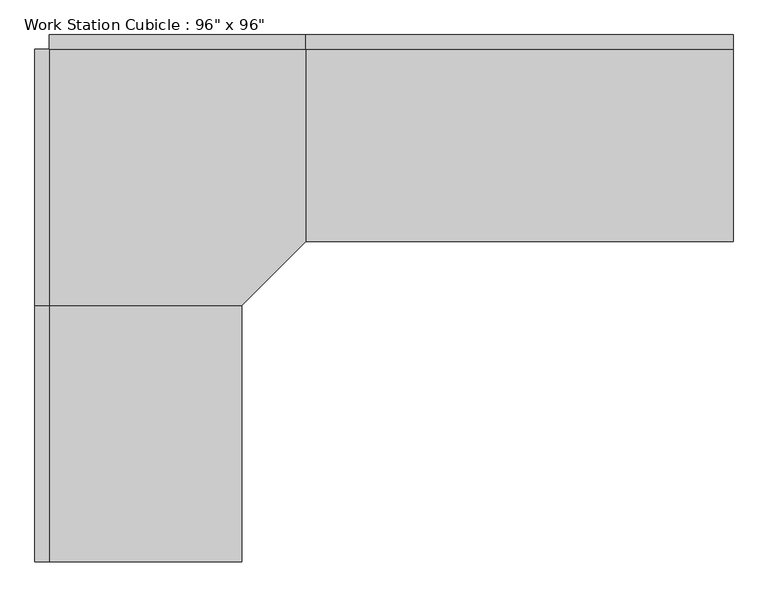
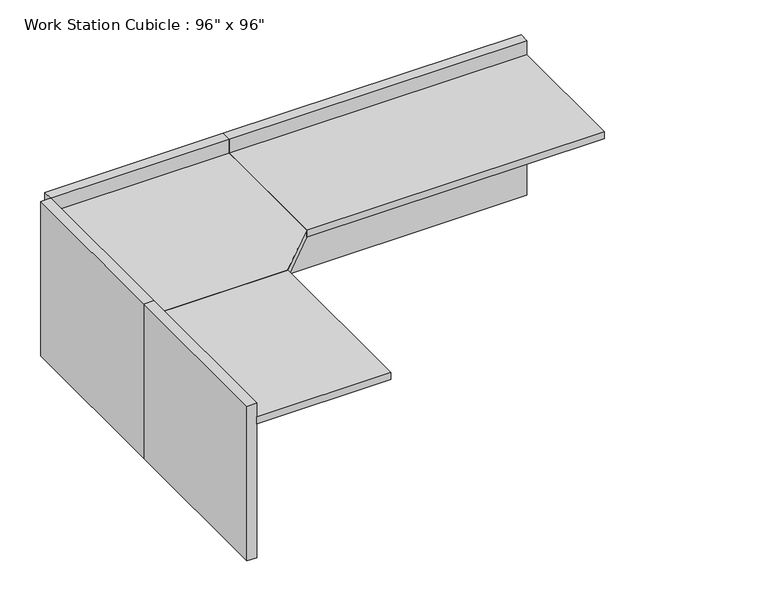
"""IFC4 building model written with IfcOpenShell, lengths in millimetres: furniture geometry."""

from ifc_helpers import new_model, si_unit, frame, origin, origin_with_axes, place, context, project, spatial, polyline, outline, extrude, source, transform, mapped, element, save


def furniture_9653231d(model_context):
    return source(origin(), model_context, "Body", "SweptSolid", [
        extrude(outline(polyline([(-80.9317522, -545.8230076), (833.4682478, -545.8230076), (833.4682478, -1231.6230076), (604.8682478, -1460.2230076), (-80.9317522, -1460.2230076), (-80.9317522, -545.8230076)])), frame((0.0, 0.0, 723.9), z_axis=(0.0, 0.0, 1.0), x_axis=(1.0, 0.0, 0.0)), (0.0, 0.0, 1.0), 38.1),
        extrude(outline(polyline([(604.8682478, -2374.6230076), (-80.9317522, -2374.6230076), (-80.9317522, -1460.2230076), (604.8682478, -1460.2230076), (604.8682478, -2374.6230076)])), frame((0.0, 0.0, 723.9), z_axis=(0.0, 0.0, 1.0), x_axis=(1.0, 0.0, 0.0)), (0.0, 0.0, 1.0), 38.1),
        extrude(outline(polyline([(2357.4682478, -1231.6230076), (833.4682478, -1231.6230076), (833.4682478, -545.8230076), (2357.4682478, -545.8230076), (2357.4682478, -1231.6230076)])), frame((0.0, 0.0, 723.9), z_axis=(0.0, 0.0, 1.0), x_axis=(1.0, 0.0, 0.0)), (0.0, 0.0, 1.0), 38.1),
        extrude(outline(polyline([(2357.4682478, -545.8230076), (833.4682478, -545.8230076), (833.4682478, -495.0230076), (2357.4682478, -495.0230076), (2357.4682478, -545.8230076)])), origin_with_axes(), (0.0, 0.0, 1.0), 838.2),
        extrude(outline(polyline([(833.4682478, -545.8230076), (-80.9317522, -545.8230076), (-80.9317522, -495.0230076), (833.4682478, -495.0230076), (833.4682478, -545.8230076)])), origin_with_axes(), (0.0, 0.0, 1.0), 838.2),
        extrude(outline(polyline([(-80.9317522, -1460.2230076), (-131.7317522, -1460.2230076), (-131.7317522, -545.8230076), (-80.9317522, -545.8230076), (-80.9317522, -1460.2230076)])), origin_with_axes(), (0.0, 0.0, 1.0), 838.2),
        extrude(outline(polyline([(-80.9317522, -2374.6230076), (-131.7317522, -2374.6230076), (-131.7317522, -1460.2230076), (-80.9317522, -1460.2230076), (-80.9317522, -2374.6230076)])), origin_with_axes(), (0.0, 0.0, 1.0), 838.2),
    ])


if __name__ == "__main__":
    model = new_model("IFC4")
    model_context = context("Model", 3, world=origin())
    ifc_project = project(units=[si_unit("LENGTHUNIT", "METRE", prefix="MILLI")], contexts=[model_context])
    site = spatial("IfcSite", under=ifc_project)
    building = spatial("IfcBuilding", under=site)
    placement = place(None, origin())
    furniture_shape = furniture_9653231d(model_context)
    element("IfcFurniture", 1, ObjectType="Work Station Cubicle : 96\" x 96\"", at=placement, inside=building, context=model_context, shape_type="MappedRepresentation", body=[
        mapped(furniture_shape, transform((0.0, 0.0, 0.0), x_axis=(1.0, 0.0, 0.0), y_axis=(0.0, 1.0, 0.0), z_axis=(0.0, 0.0, 1.0))),
    ])
    save(model, "model.ifc")

# Revit data of these elements
# Type "Work Station Cubicle : 96\" x 96\""
#   Assembly Code = "E2020"
#   Desktop Height = 2' - 6"
#   Desktop1 Width = 2' - 3"
#   Desktop2 Width = 2' - 3"
#   Panel Height = 2' - 9"
#   Panel1 Length = 3' - 0"
#   Panel2 Length = 5' - 0"
#   Cube Panel Material = Textile - Light Gray
#   Work Top Material = Laminate, Ivory, Matte
#   Default Elevation = 0
# Element 1 (IfcFurniture, "Work Station Cubicle : 96\" x 96\"")
#   Materials on its faces: "Textile - Light Gray", "Laminate, Ivory, Matte"
# Materials
#   "Textile - Light Gray": class "Fabric", colour RGB 204 204 204, transparency 0
#   "Laminate, Ivory, Matte": class "Plastic", colour RGB 247 247 239, transparency 0, Description = "Plastic Laminate - Ivory, Matte", Cost = 0
